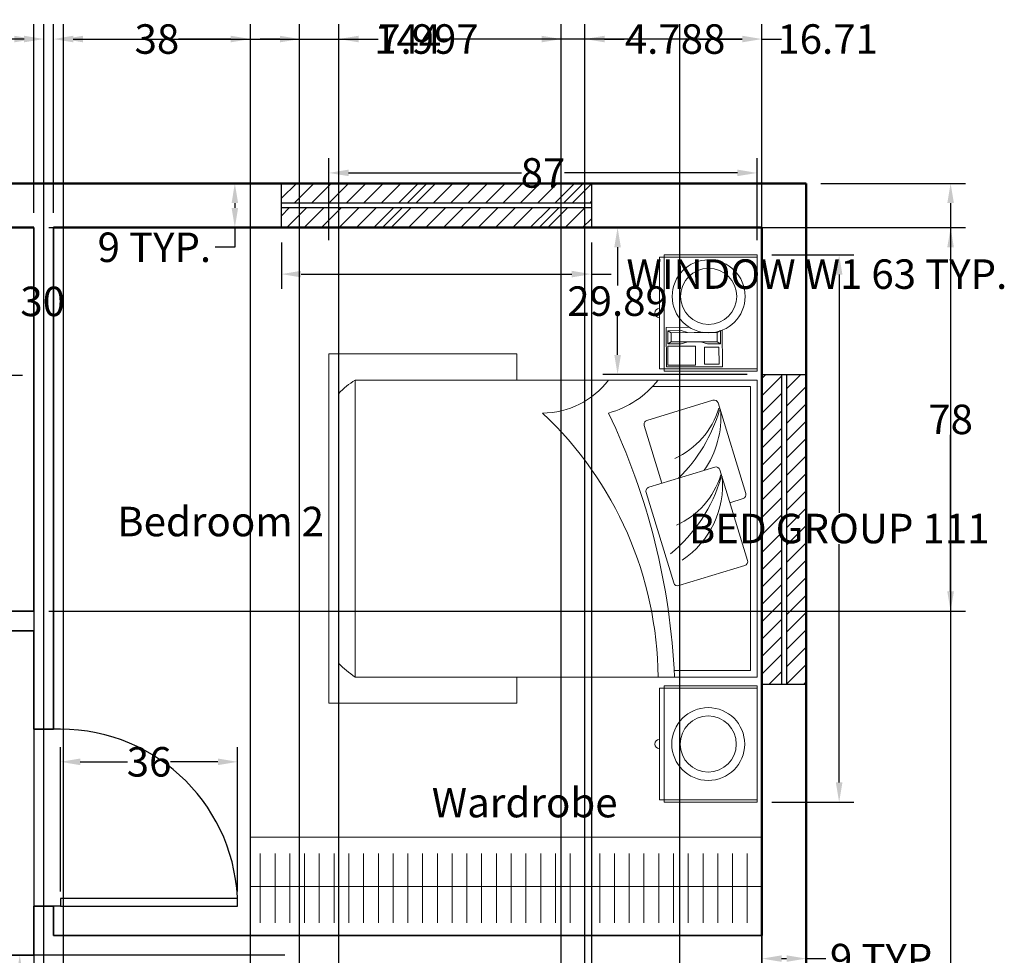
# Model space of a CAD drawing. Units: inches. Extents: x -1285 to -837, y -84 to 552.
# Tile 10 of 10: x -1037 to -837, y 362 to 552. Entities that reach past the tile are written whole.
import ezdxf

# ---------------------------------------------------------------- set-up
doc = ezdxf.new("R2010")
doc.units = ezdxf.units.IN
doc.header["$MEASUREMENT"] = 0
for name, color, linetype, lineweight in [('A-ANNO-DIMS', 2, 'Continuous', 18), ('A-ANNO-TEXT', 7, 'Continuous', 18), ('A-AREA-IDEN', 7, 'Continuous', 25), ('A-GLAZ-PATT', 191, 'Continuous', 13), ('Beds', 74, 'Continuous', 18), ('Doors', 34, 'Continuous', 25), ('Inner Wall', 202, 'Continuous', 35), ('Outer Wall', 12, 'Continuous', 50), ('Wardrobe', 145, 'Continuous', 18), ('Windows', 191, 'Continuous', 25)]:
    doc.layers.add(name, color=color, linetype=linetype, lineweight=lineweight)
doc.styles.get("Standard").update_dxf_attribs({"font": 'arial.ttf'})
doc.dimstyles.get("Standard").update_dxf_attribs({"dimtxt": 6, "dimasz": 4, "dimexe": 3, "dimexo": 3, "dimgap": 0.09, "dimtad": 0, "dimtih": 1, "dimtoh": 1, "dimdec": 1, "dimzin": 0, "dimdsep": 46, "dimlunit": 3, "dimtxsty": 'Standard', "dimcen": 0.09, "dimadec": 0, "dimazin": 0, "dimtfac": 1, "dimtdec": 1, "dimtofl": 0, "dimtmove": 0, "dimatfit": 3, "dimfxl": 1, "dimtolj": 1, "dimtzin": 0, "dimarcsym": 0})

# ---------------------------------------------------------------- blocks, each defined once
blk = doc.blocks.new('Double bed')
for p, q in [((1422.016, 1006.492), (1422.016, 1015.393)), ((1422.016, 1015.393), (1433.142, 1015.393)), ((1422.239, 1006.047), (1422.239, 1015.393)), ((1432.92, 1015.393), (1432.92, 1006.047)), ((1433.142, 1015.393), (1433.142, 1006.492)), ((1433.999, 1015.393), (1433.999, 1005.908)), ((1462.453, 1015.393), (1433.999, 1015.393)), ((1462.453, 1007.489), (1462.453, 1015.393)), ((1463.309, 1015.393), (1463.309, 1006.491)), ((1474.436, 1015.393), (1463.309, 1015.393)), ((1463.531, 1015.393), (1463.531, 1006.046)), ((1474.214, 1006.046), (1474.214, 1015.393)), ((1474.436, 1006.491), (1474.436, 1015.393)), ((1444.87, 1014.313), (1436.198, 1011.659)), ((1451.273, 1014.487), (1442.6, 1011.833)), ((1445.364, 1014.05), (1445.748, 1012.796)), ((1451.766, 1014.225), (1453.699, 1007.909)), ((1432.723, 1012.072), (1429.217, 1012.059)), ((1429.252, 1011.901), (1430.515, 1011.906)), ((1429.443, 1011.586), (1429.252, 1011.901)), ((1430.515, 1011.906), (1430.327, 1011.589)), ((1430.515, 1011.906), (1430.52, 1010.643)), ((1432.743, 1006.707), (1432.723, 1012.072)), ((1429.443, 1011.586), (1430.327, 1011.589)), ((1429.451, 1009.377), (1429.443, 1011.586)), ((1430.335, 1009.38), (1430.327, 1011.589)), ((1435.935, 1011.165), (1437.868, 1004.85)), ((1442.338, 1011.34), (1444.27, 1005.024)), ((1429.411, 1010.132), (1429.449, 1010.008)), ((1430.52, 1010.643), (1430.333, 1010.011)), ((1429.451, 1009.377), (1429.46, 1007.168)), ((1430.335, 1009.38), (1430.343, 1007.171)), ((1428.948, 1008.926), (1428.957, 1006.693)), ((1429.267, 1008.114), (1429.454, 1008.746)), ((1429.272, 1006.852), (1429.267, 1008.114)), ((1430.529, 1008.119), (1430.337, 1008.749)), ((1430.534, 1006.856), (1430.529, 1008.119)), ((1429.46, 1007.168), (1429.272, 1006.852)), ((1429.46, 1007.168), (1430.343, 1007.171)), ((1430.534, 1006.856), (1430.343, 1007.171)), ((1453.437, 1007.416), (1444.764, 1004.762)), ((1462.453, 1007.489), (1462.453, 976.891)), ((1433.142, 1006.492), (1422.016, 1006.492)), ((1428.957, 1006.693), (1432.743, 1006.707)), ((1429.272, 1006.852), (1430.534, 1006.856)), ((1443.887, 1006.278), (1438.362, 1004.587)), ((1463.309, 1006.491), (1474.436, 1006.491)), ((1432.92, 1006.047), (1422.239, 1006.047)), ((1433.999, 1005.908), (1433.999, 976.891)), ((1463.531, 1006.046), (1474.214, 1006.046)), ((1431.499, 992.391), (1431.499, 974.391)), ((1431.499, 992.391), (1433.999, 992.391)), ((1462.453, 992.391), (1464.953, 992.391)), ((1464.953, 992.391), (1464.953, 974.391)), ((1433.999, 976.891), (1462.453, 976.891)), ((1435.277, 975.333), (1461.153, 975.333)), ((1431.499, 974.391), (1464.953, 974.391))]:
    blk.add_line(p, q)
blk.add_lwpolyline([(1461.821, 1007.458), (1461.821, 1014.761), (1434.631, 1014.761), (1434.631, 1005.368)])
for points in [[(1430.847, 1011.749), (1430.852, 1010.361), (1432.493, 1010.367), (1432.488, 1011.755)], [(1430.745, 1009.508), (1430.755, 1006.857), (1432.585, 1006.864), (1432.575, 1009.515)]]:
    blk.add_lwpolyline(points, close=True)
for points in [[(1433.999, 1005.908, -0.162278), (1437.16, 1001.166, -0.100664), (1462.453, 1007.489, -0.100664)], [(1433.999, 1001.166, -0.236068), (1437.16, 994.843, -0.205258), (1462.453, 1005.908, -0.205258)]]:
    blk.add_lwpolyline(points, format="xyb")
for centre, radius in [((1425.979, 1010.759), 3.489), ((1468.873, 1010.72), 3.49), ((1425.979, 1010.759), 2.689), ((1468.873, 1010.72), 2.688)]:
    blk.add_circle(centre, radius)
for centre, radius, start, end in [((1444.986, 1013.935), 0.395, 17.0142, 107.0142), ((1451.389, 1014.109), 0.395, 17.0142, 107.0142), ((1437.622, 1003.224), 8.697, 54.68511, 95.16051), ((1442.716, 1011.455), 0.395, 107.0142, 197.0142), ((1440.838, 1004.506), 7.75, 24.22087, 73.06906), ((1444.025, 1003.399), 8.697, 33.78007, 95.16051), ((1439.066, 997.582), 14.992, 39.40233, 73.71889), ((1436.313, 1011.281), 0.395, 107.0142, 197.0142), ((1434.436, 1004.331), 7.75, 24.22087, 73.06906), ((1432.664, 997.407), 14.992, 44.27274, 73.71889), ((1453.321, 1007.794), 0.395, 287.0142, 17.0142), ((1427.579, 1006.047), 0.445, 180, 0), ((1468.873, 1006.046), 0.445, 180, 0), ((1438.246, 1004.965), 0.395, 197.0142, 287.0142), ((1444.648, 1005.14), 0.395, 197.0142, 287.0142), ((1441.427, 981.679), 8.838, 212.80295, 225.90033), ((1453.915, 982.69), 10.321, 314.52979, 325.81583)]:
    blk.add_arc(centre, radius, start, end)
blk = doc.blocks.new('*U15')
for p, q in [((0, 0), (0, 6)), ((40, 0), (40, 6))]:
    blk.add_line(p, q)
blk.add_lwpolyline([(0, 0), (0, -40), (1.75, -40), (1.75, 0)], close=True)
blk.add_arc((0, 0), 40, 270, 0)
blk = doc.blocks.new('WIN-63x9')
for p, q in [((4, 63.04), (4, 0)), ((5, 63.04), (5, 0))]:
    blk.add_line(p, q)
blk.add_lwpolyline([(0, 0), (0, 63.04), (9, 63.04), (9, 0)], close=True)
blk = doc.blocks.new('*D29')
at = {"layer": 'A-ANNO-DIMS', "color": 0, "lineweight": -2, "transparency": 16777216}
for p, q in [((-984.23, 506.94), (-984.23, 497.48)), ((-921.19, 506.94), (-921.19, 497.48)), ((-980.23, 500.48), (-925.19, 500.48)), ((-921.19, 500.48), (-917.19, 500.48))]:
    blk.add_line(p, q, dxfattribs=at)
at = {"layer": 'A-ANNO-DIMS', "color": 0, "transparency": 16777216}
for points in [[(-980.23, 501.15), (-980.23, 499.82), (-984.23, 500.48)], [(-925.19, 501.15), (-925.19, 499.82), (-921.19, 500.48)]]:
    blk.add_solid(points, dxfattribs=at)
at = {"layer": 'Defpoints', "color": 0, "transparency": 16777216}
for p in [(-984.23, 509.94), (-921.19, 509.94), (-921.19, 500.48)]:
    blk.add_point(p, dxfattribs=at)
at = {"layer": 'A-ANNO-DIMS', "color": 0, "transparency": 16777216, "insert": (-875.37, 500.48), "char_height": 6, "attachment_point": 5}
blk.add_mtext('\\A1;WINDOW W1 63 TYP.', dxfattribs=at)
blk = doc.blocks.new('*D30')
at = {"layer": 'A-ANNO-DIMS', "color": 0, "lineweight": -2, "transparency": 16777216}
for p, q in [((-987.23, 518.94), (-996.69, 518.94)), ((-993.69, 514.94), (-993.69, 513.94)), ((-987.23, 509.94), (-996.69, 509.94)), ((-993.69, 509.94), (-993.69, 505.94)), ((-993.69, 505.94), (-997.69, 505.94))]:
    blk.add_line(p, q, dxfattribs=at)
at = {"layer": 'A-ANNO-DIMS', "color": 0, "transparency": 16777216}
for points in [[(-994.35, 514.94), (-993.02, 514.94), (-993.69, 518.94)], [(-994.35, 513.94), (-993.02, 513.94), (-993.69, 509.94)]]:
    blk.add_solid(points, dxfattribs=at)
at = {"layer": 'Defpoints', "color": 0, "transparency": 16777216}
for p in [(-984.23, 518.94), (-993.69, 509.94), (-984.23, 509.94)]:
    blk.add_point(p, dxfattribs=at)
at = {"layer": 'A-ANNO-DIMS', "color": 0, "transparency": 16777216, "insert": (-1010.05, 505.94), "char_height": 6, "attachment_point": 5}
blk.add_mtext('\\A1;9 TYP.', dxfattribs=at)
blk = doc.blocks.new('*D32')
at = {"layer": 'A-ANNO-DIMS', "color": 0, "lineweight": -2, "transparency": 16777216}
for p, q in [((-886.53, 359.12), (-886.53, 364.27)), ((-877.53, 359.12), (-877.53, 364.27)), ((-882.53, 361.27), (-881.53, 361.27)), ((-877.53, 361.27), (-873.53, 361.27))]:
    blk.add_line(p, q, dxfattribs=at)
at = {"layer": 'A-ANNO-DIMS', "color": 0, "transparency": 16777216}
for points in [[(-882.53, 361.94), (-882.53, 360.61), (-886.53, 361.27)], [(-881.53, 361.94), (-881.53, 360.61), (-877.53, 361.27)]]:
    blk.add_solid(points, dxfattribs=at)
at = {"layer": 'Defpoints', "color": 0, "transparency": 16777216}
for p in [(-877.53, 361.27), (-886.53, 356.12), (-877.53, 356.12)]:
    blk.add_point(p, dxfattribs=at)
at = {"layer": 'A-ANNO-DIMS', "color": 0, "transparency": 16777216, "insert": (-861.17, 361.27), "char_height": 6, "attachment_point": 5}
blk.add_mtext('\\A1;9 TYP.', dxfattribs=at)
blk = doc.blocks.new('*D37')
at = {"layer": 'A-ANNO-DIMS', "color": 0, "lineweight": -2, "transparency": 16777216}
for p, q in [((-1041.37, 509.94), (-1036.87, 509.94)), ((-1039.87, 505.94), (-1039.87, 498.13)), ((-1039.87, 483.93), (-1039.87, 491.74)), ((-1041.37, 479.93), (-1036.87, 479.93))]:
    blk.add_line(p, q, dxfattribs=at)
at = {"layer": 'A-ANNO-DIMS', "color": 0, "transparency": 16777216}
for points in [[(-1040.54, 505.94), (-1039.2, 505.94), (-1039.87, 509.94)], [(-1040.54, 483.93), (-1039.2, 483.93), (-1039.87, 479.93)]]:
    blk.add_solid(points, dxfattribs=at)
at = {"layer": 'Defpoints', "color": 0, "transparency": 16777216}
for p in [(-1044.37, 509.94), (-1039.87, 509.94), (-1044.37, 479.93)]:
    blk.add_point(p, dxfattribs=at)
at = {"layer": 'A-ANNO-DIMS', "color": 0, "transparency": 16777216, "insert": (-1039.87, 494.93), "char_height": 6, "attachment_point": 5}
blk.add_mtext('\\A1;WC 30', dxfattribs=at)
blk = doc.blocks.new('*D43')
at = {"layer": 'A-ANNO-DIMS', "color": 0, "lineweight": -2, "transparency": 16777216}
for p, q in [((-884.53, 504.37), (-867.84, 504.37)), ((-870.84, 500.37), (-870.84, 451.93)), ((-870.84, 397.1), (-870.84, 445.54)), ((-884.53, 393.1), (-867.84, 393.1))]:
    blk.add_line(p, q, dxfattribs=at)
at = {"layer": 'A-ANNO-DIMS', "color": 0, "transparency": 16777216}
for points in [[(-871.51, 500.37), (-870.17, 500.37), (-870.84, 504.37)], [(-871.51, 397.1), (-870.17, 397.1), (-870.84, 393.1)]]:
    blk.add_solid(points, dxfattribs=at)
at = {"layer": 'Defpoints', "color": 0, "transparency": 16777216}
for p in [(-887.53, 504.37), (-887.53, 393.1), (-870.84, 393.1)]:
    blk.add_point(p, dxfattribs=at)
at = {"layer": 'A-ANNO-DIMS', "color": 0, "transparency": 16777216, "insert": (-870.84, 448.74), "char_height": 6, "attachment_point": 5}
blk.add_mtext('\\A1;BED GROUP 111', dxfattribs=at)
blk = doc.blocks.new('*D44')
at = {"layer": 'A-ANNO-DIMS', "color": 0, "lineweight": -2, "transparency": 16777216}
for p, q in [((-974.56, 507.37), (-974.56, 524.06)), ((-887.53, 507.37), (-887.53, 524.06)), ((-970.56, 521.06), (-935.44, 521.06)), ((-891.53, 521.06), (-926.66, 521.06))]:
    blk.add_line(p, q, dxfattribs=at)
at = {"layer": 'A-ANNO-DIMS', "color": 0, "transparency": 16777216}
for points in [[(-970.56, 521.73), (-970.56, 520.4), (-974.56, 521.06)], [(-891.53, 521.73), (-891.53, 520.4), (-887.53, 521.06)]]:
    blk.add_solid(points, dxfattribs=at)
at = {"layer": 'Defpoints', "color": 0, "transparency": 16777216}
for p in [(-887.53, 521.06), (-974.56, 504.37), (-887.53, 504.37)]:
    blk.add_point(p, dxfattribs=at)
at = {"layer": 'A-ANNO-DIMS', "color": 0, "transparency": 16777216, "insert": (-931.05, 521.06), "char_height": 6, "attachment_point": 5}
blk.add_mtext('\\A1;87', dxfattribs=at)
blk = doc.blocks.new('*D65')
at = {"layer": 'A-ANNO-DIMS', "color": 0, "lineweight": -2, "transparency": 16777216}
for p, q in [((-1064.13, 361.96), (-1034.42, 361.96)), ((-1037.42, 357.96), (-1037.42, 266.12)), ((-1037.42, 167.9), (-1037.42, 259.73)), ((-1064.13, 163.9), (-1034.42, 163.9))]:
    blk.add_line(p, q, dxfattribs=at)
at = {"layer": 'A-ANNO-DIMS', "color": 0, "transparency": 16777216}
for points in [[(-1038.09, 357.96), (-1036.75, 357.96), (-1037.42, 361.96)], [(-1038.09, 167.9), (-1036.75, 167.9), (-1037.42, 163.9)]]:
    blk.add_solid(points, dxfattribs=at)
at = {"layer": 'Defpoints', "color": 0, "transparency": 16777216}
for p in [(-1067.13, 361.96), (-1037.42, 361.96), (-1067.13, 163.9)]:
    blk.add_point(p, dxfattribs=at)
at = {"layer": 'A-ANNO-DIMS', "color": 0, "transparency": 16777216, "insert": (-1037.42, 262.93), "char_height": 6, "attachment_point": 5}
blk.add_mtext('\\A1;LOUNGE GROUP 198', dxfattribs=at)
blk = doc.blocks.new('*D70')
at = {"layer": 'A-ANNO-DIMS', "color": 0, "lineweight": -2, "transparency": 16777216}
for p, q in [((-874.53, 518.94), (-845.18, 518.94)), ((-848.18, 514.94), (-848.18, 237.09)), ((-848.18, -47.06), (-848.18, 230.79)), ((-874.53, -51.06), (-845.18, -51.06))]:
    blk.add_line(p, q, dxfattribs=at)
at = {"layer": 'A-ANNO-DIMS', "color": 0, "transparency": 16777216}
for points in [[(-848.85, 514.94), (-847.51, 514.94), (-848.18, 518.94)], [(-848.85, -47.06), (-847.51, -47.06), (-848.18, -51.06)]]:
    blk.add_solid(points, dxfattribs=at)
at = {"layer": 'Defpoints', "color": 0, "transparency": 16777216}
for p in [(-877.53, 518.94), (-848.18, 518.94), (-877.53, -51.06)]:
    blk.add_point(p, dxfattribs=at)
at = {"layer": 'A-ANNO-DIMS', "color": 0, "transparency": 16777216, "insert": (-848.18, 233.94), "char_height": 6, "attachment_point": 5}
blk.add_mtext('\\A1;570', dxfattribs=at)
blk = doc.blocks.new('*D72')
at = {"layer": 'A-ANNO-DIMS', "color": 0, "lineweight": -2, "transparency": 16777216}
for p, q in [((-1088.53, 512.94), (-1088.53, 551.29)), ((-1034.53, 512.94), (-1034.53, 551.29)), ((-1084.53, 548.29), (-1065.9, 548.29)), ((-1038.53, 548.29), (-1057.15, 548.29))]:
    blk.add_line(p, q, dxfattribs=at)
at = {"layer": 'A-ANNO-DIMS', "color": 0, "transparency": 16777216}
for points in [[(-1084.53, 548.96), (-1084.53, 547.62), (-1088.53, 548.29)], [(-1038.53, 548.96), (-1038.53, 547.62), (-1034.53, 548.29)]]:
    blk.add_solid(points, dxfattribs=at)
at = {"layer": 'Defpoints', "color": 0, "transparency": 16777216}
for p in [(-1034.53, 548.29), (-1088.53, 509.94), (-1034.53, 509.94)]:
    blk.add_point(p, dxfattribs=at)
at = {"layer": 'A-ANNO-DIMS', "color": 0, "transparency": 16777216, "insert": (-1061.53, 548.29), "char_height": 6, "attachment_point": 5}
blk.add_mtext('\\A1;54', dxfattribs=at)
blk = doc.blocks.new('*D73')
at = {"layer": 'A-ANNO-DIMS', "color": 0, "lineweight": -2, "transparency": 16777216}
for p, q in [((-1030.53, 512.94), (-1030.53, 551.29)), ((-886.53, 512.94), (-886.53, 551.29)), ((-1026.53, 548.29), (-964.95, 548.29)), ((-890.53, 548.29), (-952.11, 548.29))]:
    blk.add_line(p, q, dxfattribs=at)
at = {"layer": 'A-ANNO-DIMS', "color": 0, "transparency": 16777216}
for points in [[(-1026.53, 548.96), (-1026.53, 547.62), (-1030.53, 548.29)], [(-890.53, 548.96), (-890.53, 547.62), (-886.53, 548.29)]]:
    blk.add_solid(points, dxfattribs=at)
at = {"layer": 'Defpoints', "color": 0, "transparency": 16777216}
for p in [(-886.53, 548.29), (-1030.53, 509.94), (-886.53, 509.94)]:
    blk.add_point(p, dxfattribs=at)
at = {"layer": 'A-ANNO-DIMS', "color": 0, "transparency": 16777216, "insert": (-958.53, 548.29), "char_height": 6, "attachment_point": 5}
blk.add_mtext('\\A1;144', dxfattribs=at)
blk = doc.blocks.new('*D80')
at = {"layer": 'A-ANNO-DIMS', "color": 0, "lineweight": -2, "transparency": 16777216}
for p, q in [((-1184.53, -13.66), (-1184.53, 551.29)), ((-1032.53, -13.66), (-1032.53, 551.29)), ((-1180.53, 548.29), (-1114.94, 548.29)), ((-1036.53, 548.29), (-1102.12, 548.29))]:
    blk.add_line(p, q, dxfattribs=at)
at = {"layer": 'A-ANNO-DIMS', "color": 0, "transparency": 16777216}
for points in [[(-1180.53, 548.96), (-1180.53, 547.62), (-1184.53, 548.29)], [(-1036.53, 548.96), (-1036.53, 547.62), (-1032.53, 548.29)]]:
    blk.add_solid(points, dxfattribs=at)
at = {"layer": 'Defpoints', "color": 0, "transparency": 16777216}
for p in [(-1032.53, 548.29), (-1184.53, -16.66), (-1032.53, -16.66)]:
    blk.add_point(p, dxfattribs=at)
at = {"layer": 'A-ANNO-DIMS', "color": 0, "transparency": 16777216, "insert": (-1108.53, 548.29), "char_height": 6, "attachment_point": 5}
blk.add_mtext('\\A1;152', dxfattribs=at)
blk = doc.blocks.new('*D83')
at = {"layer": 'A-ANNO-DIMS', "color": 0, "lineweight": -2, "transparency": 16777216}
for p, q in [((-1031.53, 509.94), (-845.18, 509.94)), ((-848.18, 505.94), (-848.18, 474.09)), ((-848.18, 435.94), (-848.18, 467.79)), ((-1031.53, 431.94), (-845.18, 431.94))]:
    blk.add_line(p, q, dxfattribs=at)
at = {"layer": 'A-ANNO-DIMS', "color": 0, "transparency": 16777216}
for points in [[(-848.85, 505.94), (-847.51, 505.94), (-848.18, 509.94)], [(-848.85, 435.94), (-847.51, 435.94), (-848.18, 431.94)]]:
    blk.add_solid(points, dxfattribs=at)
at = {"layer": 'Defpoints', "color": 0, "transparency": 16777216}
for p in [(-1034.53, 509.94), (-848.18, 509.94), (-1034.53, 431.94)]:
    blk.add_point(p, dxfattribs=at)
at = {"layer": 'A-ANNO-DIMS', "color": 0, "transparency": 16777216, "insert": (-848.18, 470.94), "char_height": 6, "attachment_point": 5}
blk.add_mtext('\\A1;78', dxfattribs=at)
blk = doc.blocks.new('*D91')
at = {"layer": 'A-ANNO-DIMS', "color": 0, "lineweight": -2, "transparency": 16777216}
for p, q in [((-1029.13, 374.94), (-1029.13, 404.29)), ((-993.13, 374.94), (-993.13, 404.29)), ((-1025.13, 401.29), (-1015.51, 401.29)), ((-997.13, 401.29), (-1006.75, 401.29))]:
    blk.add_line(p, q, dxfattribs=at)
at = {"layer": 'A-ANNO-DIMS', "color": 0, "transparency": 16777216}
for points in [[(-1025.13, 401.96), (-1025.13, 400.62), (-1029.13, 401.29)], [(-997.13, 401.96), (-997.13, 400.62), (-993.13, 401.29)]]:
    blk.add_solid(points, dxfattribs=at)
at = {"layer": 'Defpoints', "color": 0, "transparency": 16777216}
for p in [(-993.13, 401.29), (-1029.13, 371.94), (-993.13, 371.94)]:
    blk.add_point(p, dxfattribs=at)
at = {"layer": 'A-ANNO-DIMS', "color": 0, "transparency": 16777216, "insert": (-1011.13, 401.29), "char_height": 6, "attachment_point": 5}
blk.add_mtext('\\A1;36', dxfattribs=at)
blk = doc.blocks.new('*D93')
at = {"layer": 'A-ANNO-DIMS', "color": 0, "lineweight": -2, "transparency": 16777216}
for p, q in [((-1028.53, 78.94), (-1028.53, 551.29)), ((-990.53, 78.94), (-990.53, 551.29)), ((-1024.53, 548.29), (-1013.92, 548.29)), ((-994.53, 548.29), (-1005.14, 548.29))]:
    blk.add_line(p, q, dxfattribs=at)
at = {"layer": 'A-ANNO-DIMS', "color": 0, "transparency": 16777216}
for points in [[(-1024.53, 548.96), (-1024.53, 547.62), (-1028.53, 548.29)], [(-994.53, 548.96), (-994.53, 547.62), (-990.53, 548.29)]]:
    blk.add_solid(points, dxfattribs=at)
at = {"layer": 'Defpoints', "color": 0, "transparency": 16777216}
for p in [(-990.53, 548.29), (-1028.53, 75.94), (-990.53, 75.94)]:
    blk.add_point(p, dxfattribs=at)
at = {"layer": 'A-ANNO-DIMS', "color": 0, "transparency": 16777216, "insert": (-1009.53, 548.29), "char_height": 6, "attachment_point": 5}
blk.add_mtext('\\A1;38', dxfattribs=at)
blk = doc.blocks.new('*D97')
at = {"layer": 'A-ANNO-DIMS', "color": 0, "lineweight": -2, "transparency": 16777216}
for p, q in [((-921.19, 506.94), (-921.19, -83.53)), ((-886.53, 506.94), (-886.53, -83.53)), ((-917.19, -80.53), (-916.43, -80.53)), ((-890.53, -80.53), (-891.3, -80.53))]:
    blk.add_line(p, q, dxfattribs=at)
at = {"layer": 'A-ANNO-DIMS', "color": 0, "transparency": 16777216}
for points in [[(-917.19, -79.86), (-917.19, -81.2), (-921.19, -80.53)], [(-890.53, -79.86), (-890.53, -81.2), (-886.53, -80.53)]]:
    blk.add_solid(points, dxfattribs=at)
at = {"layer": 'Defpoints', "color": 0, "transparency": 16777216}
for p in [(-921.19, 509.94), (-886.53, 509.94), (-886.53, -80.53)]:
    blk.add_point(p, dxfattribs=at)
at = {"layer": 'A-ANNO-DIMS', "color": 0, "transparency": 16777216, "insert": (-903.86, -80.53), "char_height": 6, "attachment_point": 5}
blk.add_mtext('\\A1;34.665', dxfattribs=at)
blk = doc.blocks.new('*D98')
at = {"layer": 'A-ANNO-DIMS', "color": 0, "lineweight": -2, "transparency": 16777216}
for p, q in [((-889.53, 509.94), (-918.88, 509.94)), ((-915.88, 505.94), (-915.88, 498.15)), ((-915.88, 484.05), (-915.88, 491.84)), ((-889.53, 480.05), (-918.88, 480.05))]:
    blk.add_line(p, q, dxfattribs=at)
at = {"layer": 'A-ANNO-DIMS', "color": 0, "transparency": 16777216}
for points in [[(-916.55, 505.94), (-915.21, 505.94), (-915.88, 509.94)], [(-916.55, 484.05), (-915.21, 484.05), (-915.88, 480.05)]]:
    blk.add_solid(points, dxfattribs=at)
at = {"layer": 'Defpoints', "color": 0, "transparency": 16777216}
for p in [(-915.88, 509.94), (-886.53, 509.94), (-886.53, 480.05)]:
    blk.add_point(p, dxfattribs=at)
at = {"layer": 'A-ANNO-DIMS', "color": 0, "transparency": 16777216, "insert": (-915.88, 494.99), "char_height": 6, "attachment_point": 5}
blk.add_mtext('\\A1;29.89', dxfattribs=at)
blk = doc.blocks.new('*D102')
at = {"layer": 'A-ANNO-DIMS', "color": 0, "lineweight": -2, "transparency": 16777216}
for p, q in [((-903.24, -39.06), (-903.24, 551.29)), ((-886.53, -39.06), (-886.53, 551.29)), ((-899.24, 548.29), (-890.53, 548.29)), ((-886.53, 548.29), (-882.53, 548.29))]:
    blk.add_line(p, q, dxfattribs=at)
at = {"layer": 'A-ANNO-DIMS', "color": 0, "transparency": 16777216}
for points in [[(-899.24, 548.96), (-899.24, 547.62), (-903.24, 548.29)], [(-890.53, 548.96), (-890.53, 547.62), (-886.53, 548.29)]]:
    blk.add_solid(points, dxfattribs=at)
at = {"layer": 'Defpoints', "color": 0, "transparency": 16777216}
for p in [(-886.53, 548.29), (-903.24, -42.06), (-886.53, -42.06)]:
    blk.add_point(p, dxfattribs=at)
at = {"layer": 'A-ANNO-DIMS', "color": 0, "transparency": 16777216, "insert": (-873.18, 548.29), "char_height": 6, "attachment_point": 5}
blk.add_mtext('\\A1;16.71', dxfattribs=at)
blk = doc.blocks.new('*D104')
at = {"layer": 'A-ANNO-DIMS', "color": 0, "lineweight": -2, "transparency": 16777216}
for p, q in [((-1044.37, 506.94), (-1044.37, -83.53)), ((-1034.53, 506.94), (-1034.53, -83.53)), ((-1040.37, -80.53), (-1038.53, -80.53)), ((-1034.53, -80.53), (-1030.53, -80.53))]:
    blk.add_line(p, q, dxfattribs=at)
at = {"layer": 'A-ANNO-DIMS', "color": 0, "transparency": 16777216}
for points in [[(-1040.37, -79.86), (-1040.37, -81.2), (-1044.37, -80.53)], [(-1038.53, -79.86), (-1038.53, -81.2), (-1034.53, -80.53)]]:
    blk.add_solid(points, dxfattribs=at)
at = {"layer": 'Defpoints', "color": 0, "transparency": 16777216}
for p in [(-1044.37, 509.94), (-1034.53, 509.94), (-1034.53, -80.53)]:
    blk.add_point(p, dxfattribs=at)
at = {"layer": 'A-ANNO-DIMS', "color": 0, "transparency": 16777216, "insert": (-1022.66, -80.53), "char_height": 6, "attachment_point": 5}
blk.add_mtext('\\A1;9.84', dxfattribs=at)
blk = doc.blocks.new('*D106')
at = {"layer": 'A-ANNO-DIMS', "color": 0, "lineweight": -2, "transparency": 16777216}
for p, q in [((-1274.88, 365.94), (-1274.88, 369.94)), ((-1274.88, 369.94), (-1270.88, 369.94)), ((-983.53, 361.94), (-1277.88, 361.94)), ((-983.53, 355.94), (-1277.88, 355.94)), ((-1274.88, 351.94), (-1274.88, 347.94))]:
    blk.add_line(p, q, dxfattribs=at)
at = {"layer": 'A-ANNO-DIMS', "color": 0, "transparency": 16777216}
for points in [[(-1275.55, 365.94), (-1274.21, 365.94), (-1274.88, 361.94)], [(-1275.55, 351.94), (-1274.21, 351.94), (-1274.88, 355.94)]]:
    blk.add_solid(points, dxfattribs=at)
at = {"layer": 'Defpoints', "color": 0, "transparency": 16777216}
for p in [(-1274.88, 361.94), (-980.53, 361.94), (-980.53, 355.94)]:
    blk.add_point(p, dxfattribs=at)
at = {"layer": 'A-ANNO-DIMS', "color": 0, "transparency": 16777216, "insert": (-1268.81, 369.94), "char_height": 6, "attachment_point": 5}
blk.add_mtext('\\A1;6', dxfattribs=at)
blk = doc.blocks.new('*D107')
at = {"layer": 'A-ANNO-DIMS', "color": 0, "lineweight": -2, "transparency": 16777216}
for p, q in [((-980.53, 316.94), (-980.53, 551.29)), ((-972.53, 317.04), (-972.53, 551.29)), ((-984.53, 548.29), (-988.53, 548.29)), ((-968.53, 548.29), (-964.53, 548.29))]:
    blk.add_line(p, q, dxfattribs=at)
at = {"layer": 'A-ANNO-DIMS', "color": 0, "transparency": 16777216}
for points in [[(-984.53, 548.96), (-984.53, 547.62), (-980.53, 548.29)], [(-968.53, 548.96), (-968.53, 547.62), (-972.53, 548.29)]]:
    blk.add_solid(points, dxfattribs=at)
at = {"layer": 'Defpoints', "color": 0, "transparency": 16777216}
for p in [(-972.53, 548.29), (-980.53, 313.94), (-972.53, 314.04)]:
    blk.add_point(p, dxfattribs=at)
at = {"layer": 'A-ANNO-DIMS', "color": 0, "transparency": 16777216, "insert": (-954.34, 548.29), "char_height": 6, "attachment_point": 5}
blk.add_mtext('\\A1;7.997', dxfattribs=at)
blk = doc.blocks.new('*D108')
at = {"layer": 'A-ANNO-DIMS', "color": 0, "lineweight": -2, "transparency": 16777216}
for p, q in [((-927.32, 316.94), (-927.32, 551.29)), ((-922.53, 316.94), (-922.53, 551.29)), ((-931.32, 548.29), (-935.32, 548.29)), ((-918.53, 548.29), (-914.53, 548.29))]:
    blk.add_line(p, q, dxfattribs=at)
at = {"layer": 'A-ANNO-DIMS', "color": 0, "transparency": 16777216}
for points in [[(-931.32, 548.96), (-931.32, 547.62), (-927.32, 548.29)], [(-918.53, 548.96), (-918.53, 547.62), (-922.53, 548.29)]]:
    blk.add_solid(points, dxfattribs=at)
at = {"layer": 'Defpoints', "color": 0, "transparency": 16777216}
for p in [(-922.53, 548.29), (-927.32, 313.94), (-922.53, 313.94)]:
    blk.add_point(p, dxfattribs=at)
at = {"layer": 'A-ANNO-DIMS', "color": 0, "transparency": 16777216, "insert": (-904.19, 548.29), "char_height": 6, "attachment_point": 5}
blk.add_mtext('\\A1;4.788', dxfattribs=at)

msp = doc.modelspace()

# ---------------------------------------------------------------- hatches: boundary and pattern name
at = {"layer": 'A-GLAZ-PATT'}
h = msp.add_hatch(dxfattribs=at)
h.set_pattern_fill('ANSI31', color=256, scale=20)
h.set_pattern_definition([(45, (-2191.666, -702.1458), (-1.767767, 1.767767), [])])
h.paths.add_polyline_path([(-921.1945, 518.9392), (-984.2307, 518.9392), (-984.2307, 514.9392), (-921.1945, 514.9392)])
h.paths.add_polyline_path([(-921.1945, 513.9392), (-984.2307, 513.9392), (-984.2307, 509.9392), (-921.1945, 509.9392)])
h.paths.add_polyline_path([(-877.5299, 480.0491), (-881.5299, 480.0491), (-881.5299, 417.0129), (-877.5299, 417.0129)])
h.paths.add_polyline_path([(-882.5299, 480.0491), (-886.5299, 480.0491), (-886.5299, 417.0129), (-882.5299, 417.0129)])
h.paths.add_polyline_path([(-877.5299, 356.1195), (-881.5299, 356.1195), (-881.5299, 321.7709), (-877.5299, 321.7709)])
h.paths.add_polyline_path([(-882.5299, 356.1195), (-886.5299, 356.1195), (-886.5299, 321.7709), (-882.5299, 321.7709)])
h.paths.add_polyline_path([(-1133.8033, 518.9392), (-1196.8396, 518.9392), (-1196.8396, 514.9392), (-1133.8033, 514.9392)])
h.paths.add_polyline_path([(-1133.8033, 513.9392), (-1196.8396, 513.9392), (-1196.8396, 509.9392), (-1133.8033, 509.9392)])
h.paths.add_polyline_path([(-1236.5299, 138.1751), (-1240.5299, 138.1751), (-1240.5299, 75.1388), (-1236.5299, 75.1388)])
h.paths.add_polyline_path([(-1241.5299, 138.1751), (-1245.5299, 138.1751), (-1245.5299, 75.1388), (-1241.5299, 75.1388)])
h.paths.add_polyline_path([(-1236.5299, 35.9392), (-1240.5299, 35.9392), (-1240.5299, 1.5906), (-1236.5299, 1.5906)])
h.paths.add_polyline_path([(-1241.5299, 35.9392), (-1245.5299, 35.9392), (-1245.5299, 1.5906), (-1241.5299, 1.5906)])
h.paths.add_polyline_path([(-1088.8155, -16.6608), (-1136.8155, -16.6608), (-1136.8155, -20.6608), (-1088.8155, -20.6608)])
h.paths.add_polyline_path([(-1088.8155, -21.6608), (-1136.8155, -21.6608), (-1136.8155, -25.6608), (-1088.8155, -25.6608)])
h = msp.add_hatch(dxfattribs=at)
h.set_pattern_fill('ANSI31', color=256, scale=90)
h.set_pattern_definition([(45, (-2191.666, -702.146), (-7.95495, 7.95495), [])])
h.paths.add_polyline_path([(-921.1945, 513.9392), (-984.2307, 513.9392), (-984.2307, 509.9392), (-921.1945, 509.9392)])
h.paths.add_polyline_path([(-921.1945, 518.9392), (-984.2307, 518.9392), (-984.2307, 514.9392), (-921.1945, 514.9392)])

# ---------------------------------------------------------------- linework, layer by layer
at = {"layer": 'Inner Wall'}
for p, q in [((-1034.5299, 509.9392), (-1034.5299, 431.9392)), ((-1030.5299, 509.9392), (-1030.5299, 407.9392)), ((-1040.5299, 431.9392), (-1034.5299, 431.9392)), ((-1040.5299, 427.9392), (-1034.5299, 427.9392)), ((-1034.5299, 427.9392), (-1034.5299, 407.9392)), ((-1034.5299, 407.9392), (-1030.5299, 407.9392)), ((-1034.5299, 371.9392), (-1030.5299, 371.9392)), ((-1034.5299, 371.9392), (-1034.5299, 361.9392)), ((-1030.5299, 371.9392), (-1030.5299, 365.9392)), ((-1030.5299, 365.9392), (-886.5299, 365.9392))]:
    msp.add_line(p, q, dxfattribs=at)
at = {"layer": 'Outer Wall'}
for p, q in [((-1245.5299, 518.9392), (-877.5299, 518.9392)), ((-877.5299, 518.9392), (-877.5299, -51.0608)), ((-1088.5299, 509.9392), (-1034.5299, 509.9392)), ((-1030.5299, 509.9392), (-886.5299, 509.9392)), ((-886.5299, 509.9392), (-886.5299, 365.9392))]:
    msp.add_line(p, q, dxfattribs=at)
at = {"layer": 'Wardrobe'}
for p, q in [((-988.5134, 368.5793), (-988.5134, 382.632)), ((-985.5134, 368.5793), (-985.5134, 382.632)), ((-982.5134, 368.5793), (-982.5134, 382.632)), ((-979.5134, 368.5793), (-979.5134, 382.632)), ((-976.5134, 368.5793), (-976.5134, 382.632)), ((-973.5134, 368.5793), (-973.5134, 382.632)), ((-970.5134, 368.5793), (-970.5134, 382.632)), ((-967.5134, 368.5793), (-967.5134, 382.632)), ((-964.5134, 368.5793), (-964.5134, 382.632)), ((-961.5134, 368.5793), (-961.5134, 382.632)), ((-958.5134, 368.5793), (-958.5134, 382.632)), ((-955.5134, 368.5793), (-955.5134, 382.632)), ((-952.5134, 368.5793), (-952.5134, 382.632)), ((-949.5134, 368.5793), (-949.5134, 382.632)), ((-946.5134, 368.5793), (-946.5134, 382.632)), ((-943.5134, 368.5793), (-943.5134, 382.632)), ((-940.5134, 368.5793), (-940.5134, 382.632)), ((-937.5134, 368.5793), (-937.5134, 382.632)), ((-934.5134, 368.5793), (-934.5134, 382.632)), ((-931.5134, 368.5793), (-931.5134, 382.632)), ((-928.5134, 368.5793), (-928.5134, 382.632)), ((-925.5134, 368.5793), (-925.5134, 382.632)), ((-922.5134, 368.5793), (-922.5134, 382.632)), ((-919.5134, 368.5793), (-919.5134, 382.632)), ((-916.5134, 368.5793), (-916.5134, 382.632)), ((-913.5134, 368.5793), (-913.5134, 382.632)), ((-910.5134, 368.5793), (-910.5134, 382.632)), ((-907.5134, 368.5793), (-907.5134, 382.632)), ((-904.5134, 368.5793), (-904.5134, 382.632)), ((-901.5134, 368.5793), (-901.5134, 382.632)), ((-898.5134, 368.5793), (-898.5134, 382.632)), ((-895.5134, 368.5793), (-895.5134, 382.632)), ((-892.5134, 368.5793), (-892.5134, 382.632)), ((-889.5134, 368.5793), (-889.5134, 382.632)), ((-990.5299, 375.9392), (-886.5299, 375.9392))]:
    msp.add_line(p, q, dxfattribs=at)
msp.add_lwpolyline([(-990.5299, 385.9392), (-886.5299, 385.9392), (-886.5299, 365.9392), (-990.5299, 365.9392)], close=True, dxfattribs=at)

# ---------------------------------------------------------------- block references
at = {"layer": 'Beds', "xscale": 2.122696503450097, "yscale": 2.122696503450097, "zscale": 2.122696503450097, "rotation": 270}
msp.add_blockref('Double bed', (-3042.9014, 3522.8814), dxfattribs=at)
at = {"layer": 'Doors', "xscale": 0.9, "yscale": 0.9, "zscale": 0.9, "rotation": 90}
msp.add_blockref('*U15', (-1029.1299, 371.9392), dxfattribs=at)
at = {"layer": 'Windows', "rotation": 270.0000000000002}
msp.add_blockref('WIN-63x9', (-984.2306, 518.9394), dxfattribs=at)
at = {"layer": 'Windows'}
msp.add_blockref('WIN-63x9', (-886.53, 417.013), dxfattribs=at)

# ---------------------------------------------------------------- texts
at = {"layer": 'A-ANNO-TEXT', "insert": (-953.6579, 395.9956), "char_height": 6, "attachment_point": 1}
msp.add_mtext_dynamic_manual_height_columns('Wardrobe', width=68.784729, gutter_width=1, heights=[0], dxfattribs=at)
at = {"layer": 'A-AREA-IDEN', "insert": (-1017.6087, 453.1605), "char_height": 6, "attachment_point": 1}
msp.add_mtext_dynamic_manual_height_columns('Bedroom 2', width=68.784729, gutter_width=1, heights=[0], dxfattribs=at)

# ---------------------------------------------------------------- dimensions: what is measured, and where the dimension line sits
at = {"layer": 'A-ANNO-DIMS'}
for base, p1, p2, override, picture, middle in [((-1032.5299, 548.2892), (-1184.5299, -16.6608), (-1032.5299, -16.6608), {"dimdec": 0, "dimlfac": 1, "dimrnd": 0, "dimzin": 0, "dimdsep": 46, "dimlunit": 2}, '*D80', (-1108.5299, 548.2892)), ((-1034.5299, 548.2892), (-1088.5299, 509.9392), (-1034.5299, 509.9392), {"dimdec": 0, "dimlfac": 1, "dimrnd": 0, "dimzin": 0, "dimdsep": 46, "dimlunit": 2}, '*D72', (-1061.5299, 548.2892)), ((-886.5299, 548.2892), (-1030.5299, 509.9392), (-886.5299, 509.9392), {"dimdec": 0, "dimlfac": 1, "dimrnd": 0, "dimzin": 0, "dimdsep": 46, "dimlunit": 2}, '*D73', (-958.5299, 548.2892)), ((-990.5299, 548.2892), (-1028.5299, 75.9392), (-990.5299, 75.9392), {"dimdec": 0, "dimlfac": 1, "dimrnd": 0, "dimzin": 0, "dimdsep": 46, "dimlunit": 2}, '*D93', (-1009.5299, 548.2892)), ((-972.5331, 548.2892), (-980.5299, 313.9392), (-972.5331, 314.0433), {"dimdec": 3, "dimlfac": 1, "dimrnd": 0, "dimzin": 0, "dimdsep": 46, "dimlunit": 2}, '*D107', (-954.3442, 548.2892)), ((-922.5299, 548.2892), (-927.318, 313.9392), (-922.5299, 313.9392), {"dimdec": 3, "dimlfac": 1, "dimrnd": 0, "dimzin": 0, "dimdsep": 46, "dimlunit": 2}, '*D108', (-904.1895, 548.2892)), ((-886.5299, 548.2892), (-903.24, -42.0608), (-886.5299, -42.0608), {"dimdec": 2, "dimlfac": 1, "dimrnd": 0, "dimzin": 0, "dimdsep": 46, "dimlunit": 2}, '*D102', (-873.1779, 548.2892)), ((-887.5299, 521.0631), (-974.564, 504.3724), (-887.5299, 504.3724), {"dimdec": 0, "dimlfac": 1, "dimrnd": 0, "dimzin": 0, "dimdsep": 46, "dimlunit": 2}, '*D44', (-931.0469, 521.0631)), ((-1034.5299, -80.5308), (-1044.3703, 509.9392), (-1034.5299, 509.9392), {"dimdec": 2, "dimlfac": 1, "dimrnd": 0, "dimzin": 0, "dimdsep": 46, "dimlunit": 2}, '*D104', (-1022.6595, -80.5308)), ((-886.5299, -80.5308), (-921.1945, 509.9392), (-886.5299, 509.9392), {"dimdec": 3, "dimlfac": 1, "dimrnd": 0, "dimzin": 0, "dimdsep": 46, "dimlunit": 2}, '*D97', (-903.8622, -80.5308)), ((-993.1299, 401.2892), (-1029.1299, 371.9392), (-993.1299, 371.9392), {"dimdec": 0, "dimlfac": 1, "dimrnd": 0, "dimzin": 0, "dimdsep": 46, "dimlunit": 2}, '*D91', (-1011.1299, 401.2892))]:
    dim = msp.add_linear_dim(base=base, p1=p1, p2=p2, dimstyle='Standard', override=override, dxfattribs=at)
    dim.commit()
    dim.dimension.update_dxf_attribs({"geometry": picture, "text_midpoint": middle})
for base, p1, p2, angle, text, picture, middle in [((-993.6862, 509.9392), (-984.2307, 518.9392), (-984.2307, 509.9392), 270, '<> TYP.', '*D30', (-1010.0484, 505.9392)), ((-921.1945, 500.4838), (-984.2307, 509.9392), (-921.1945, 509.9392), 0, 'WINDOW W1 <> TYP.', '*D29', (-875.3746, 500.4838)), ((-1039.8683, 509.9392), (-1044.3703, 479.9262), (-1044.3703, 509.9392), 90, 'WC <>', '*D37', (-1039.8683, 494.9327)), ((-870.8392, 393.101), (-887.5299, 504.3724), (-887.5299, 393.101), 270, 'BED GROUP <>', '*D43', (-870.8392, 448.7367)), ((-1037.4189, 361.9592), (-1067.1282, 163.8976), (-1067.1282, 361.9592), 90, 'LOUNGE GROUP <>', '*D65', (-1037.4189, 262.9284))]:
    dim = msp.add_linear_dim(base=base, p1=p1, p2=p2, angle=angle, text=text, dimstyle='Standard', override={"dimdec": 0, "dimlfac": 1, "dimrnd": 0, "dimzin": 0, "dimdsep": 46, "dimlunit": 2}, dxfattribs=at)
    dim.commit()
    dim.dimension.update_dxf_attribs({"geometry": picture, "text_midpoint": middle})
for base, p1, p2, override, picture, middle in [((-848.1799, 518.9392), (-877.5299, -51.0608), (-877.5299, 518.9392), {"dimdec": 0, "dimlfac": 1, "dimrnd": 0, "dimzin": 0, "dimdsep": 46, "dimlunit": 2}, '*D70', (-848.1799, 233.9392)), ((-848.1799, 509.9392), (-1034.5299, 431.9392), (-1034.5299, 509.9392), {"dimdec": 0, "dimlfac": 1, "dimrnd": 0, "dimzin": 0, "dimdsep": 46, "dimlunit": 2}, '*D83', (-848.1799, 470.9392)), ((-915.8799, 509.9392), (-886.5299, 480.0491), (-886.5299, 509.9392), {"dimdec": 2, "dimlfac": 1, "dimrnd": 0, "dimzin": 0, "dimdsep": 46, "dimlunit": 2}, '*D98', (-915.8799, 494.9942)), ((-1274.8799, 361.9392), (-980.5299, 355.9392), (-980.5299, 361.9392), {"dimdec": 0, "dimlfac": 1, "dimrnd": 0, "dimzin": 0, "dimdsep": 46, "dimlunit": 2}, '*D106', (-1268.809, 369.9392))]:
    dim = msp.add_linear_dim(base=base, p1=p1, p2=p2, angle=90, dimstyle='Standard', override=override, dxfattribs=at)
    dim.commit()
    dim.dimension.update_dxf_attribs({"geometry": picture, "text_midpoint": middle})
dim = msp.add_linear_dim(base=(-877.5299, 361.2718), p1=(-886.5299, 356.1195), p2=(-877.5299, 356.1195), text='<> TYP.', dimstyle='Standard', override={"dimdec": 0, "dimlfac": 1, "dimrnd": 0, "dimzin": 0, "dimdsep": 46, "dimlunit": 2}, dxfattribs=at)
dim.commit()
dim.dimension.update_dxf_attribs({"geometry": '*D32', "text_midpoint": (-861.1677, 361.2718)})

doc.saveas('drawing.dxf')
